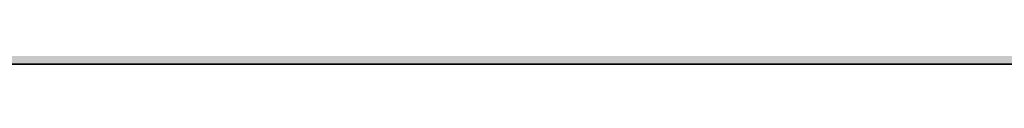
# Model space of a CAD drawing. Units: inches. Extents: x 2091 to 2899, y 967 to 2217.
# Tile 18 of 256: x 2312 to 2351, y 1091 to 1091. Entities that reach past the tile are written whole.
import ezdxf

# ---------------------------------------------------------------- set-up
doc = ezdxf.new("R2010")
doc.units = ezdxf.units.IN
doc.layers.add('A-WALL-PATT', color=141, linetype='Continuous', lineweight=13, true_color=0xadddf7)
doc.layers.add('C-PROP', color=7, linetype='Continuous', lineweight=35)

msp = doc.modelspace()

# ---------------------------------------------------------------- hatches: boundary and pattern name
at = {"layer": 'A-WALL-PATT'}
h = msp.add_hatch(color=256, dxfattribs=at)
h.dxf.hatch_style = 1
h.paths.add_polyline_path([(2212.144, 1941.419), (2387.644, 1941.419), (2387.644, 1824.419), (2392.144, 1824.419), (2392.144, 1941.419), (2609.644, 1941.419), (2609.644, 1825.919), (2614.144, 1825.919), (2614.144, 1941.419), (2794.144, 1941.419), (2794.144, 1928.762), (2803.144, 1928.762), (2803.144, 2050.919), (2203.144, 2050.919), (2203.144, 1900.758), (2212.144, 1900.758)])
h.paths.add_polyline_path([(2212.144, 1945.919), (2212.144, 2041.919), (2794.144, 2041.919), (2794.144, 1945.919), (2402.248, 1945.919), (2401.102, 1945.776), (2398.702, 1945.776)], flags=16)
h.paths.add_polyline_path([(2230.23, 1948.063), (2227.35, 1949.503), (2225.91, 1951.903), (2223.99, 1952.863), (2223.03, 1955.263), (2222.07, 1959.583), (2222.07, 1963.423), (2223.03, 1965.663), (2223.99, 1965.343), (2225.586, 1963.861), (2226.912, 1964.957), (2226.949, 1965.939), (2227.778, 1966.952), (2228.2, 1968.879), (2230.71, 1964.863), (2233.59, 1966.303), (2233.607, 1966.332), (2233.773, 1964.938), (2234.634, 1963.676), (2235.03, 1963.903), (2236.282, 1965.572), (2235.99, 1962.943), (2237.955, 1957.54), (2238.39, 1957.903), (2239.216, 1960.306), (2238.655, 1966.385), (2238.693, 1966.438), (2238.841, 1967.5), (2238.78, 1967.687), (2238.881, 1967.787), (2238.667, 1966.252), (2239.216, 1960.306), (2238.39, 1957.903), (2236.95, 1956.703), (2234.55, 1949.983)], flags=0)
h.paths.add_polyline_path([(2278.012, 1948.063), (2276.496, 1947.873), (2275.85, 1947.689), (2274.652, 1947.103)], flags=0)
h.paths.add_polyline_path([(2269.852, 1955.743), (2268.276, 1956.629), (2270.867, 1956.348), (2269.372, 1958.143), (2268.715, 1959.192), (2270.57, 1958.729), (2268.581, 1961.906), (2270.812, 1960.892), (2270.812, 1963.423), (2271.393, 1964.779), (2270.292, 1966.156), (2271.772, 1965.663), (2272.141, 1966.525), (2273.93, 1965.929), (2275.63, 1968.054), (2276.332, 1966.722), (2276.52, 1966.952), (2276.942, 1968.879), (2277.734, 1967.611), (2278.14, 1969.465), (2279.659, 1967.034), (2280.412, 1966.783), (2280.949, 1967.589), (2281.61, 1967.369), (2282.133, 1968.154), (2282.349, 1966.333), (2282.35, 1966.333), (2283.408, 1968.095), (2283.713, 1965.524), (2284.32, 1964.634), (2284.512, 1964.889), (2284.235, 1965.705), (2284.5, 1967.319), (2284.908, 1965.417), (2285.396, 1966.069), (2285.433, 1966.291), (2285.473, 1966.171), (2286.354, 1967.345), (2286.222, 1966.158), (2287.663, 1968.08), (2287.714, 1968.443), (2288.482, 1969.017), (2288.574, 1968.729), (2288.917, 1969.069), (2288.607, 1966.838), (2288.929, 1963.351), (2288.935, 1963.357), (2288.93, 1963.34), (2289.015, 1962.414), (2290.111, 1963.875), (2290.133, 1963.943), (2290.218, 1964.017), (2290.111, 1963.875), (2289.156, 1960.892), (2288.594, 1959.257), (2288.572, 1959.103), (2289.532, 1960.543), (2290.012, 1962.463), (2290.192, 1962.643), (2289.77, 1959.689), (2286.89, 1957.289), (2284.49, 1950.569), (2283.315, 1950.046), (2283.292, 1949.983), (2280.29, 1948.649), (2281.13, 1948.649), (2282.57, 1948.169), (2283.205, 1948.063), (2278.972, 1948.063), (2276.092, 1949.503), (2274.652, 1951.903), (2272.732, 1952.863)], flags=0)
h.paths.add_polyline_path([(2271.159, 1958.022), (2272.97, 1955.849), (2272.01, 1960.169), (2272.01, 1964.009), (2272.624, 1965.443), (2274.328, 1963.861), (2275.654, 1964.957), (2275.638, 1964.539), (2277.412, 1966.007), (2277.033, 1965.157), (2276.83, 1964.976), (2276.766, 1963.295), (2277.45, 1962.66), (2279.452, 1964.863), (2282.332, 1966.303), (2283.53, 1966.889), (2283.295, 1966.771), (2283.913, 1963.885), (2284.899, 1964.448), (2284.732, 1962.943), (2286.697, 1957.54), (2287.132, 1957.903), (2287.542, 1959.095), (2287.779, 1958.442), (2285.683, 1956.695), (2285.877, 1959.795), (2284.732, 1962.943), (2284.899, 1964.448), (2283.913, 1963.885), (2284.224, 1962.434), (2283.424, 1963.605), (2281.61, 1962.569), (2281.13, 1960.169), (2282.09, 1956.329), (2283.05, 1952.969), (2282.57, 1950.569), (2280.17, 1948.649), (2279.883, 1948.792), (2278.972, 1948.063), (2278.972, 1949.023), (2278.672, 1949.397), (2277.29, 1950.089), (2275.85, 1952.489), (2273.93, 1953.449), (2272.49, 1954.889), (2271.922, 1954.889), (2271.772, 1955.263)], flags=0)
h.paths.add_polyline_path([(2311.994, 1955.743), (2312.063, 1955.674), (2312.055, 1955.709)], flags=0)
h.paths.add_polyline_path([(2331.956, 1963.952), (2333.396, 1965.392), (2331.077, 1963.357), (2330.999, 1963.112)], flags=0)
h.paths.add_polyline_path([(2310.554, 1954.303), (2307.04, 1956.28), (2310.763, 1955.876), (2312.474, 1953.823), (2313.434, 1951.423), (2315.354, 1950.463), (2316.794, 1948.063), (2317.466, 1947.727), (2319.369, 1947.965), (2317.754, 1949.983), (2317.57, 1950.61), (2316.794, 1951.903), (2314.874, 1952.863), (2313.914, 1955.263), (2311.514, 1958.143), (2309.375, 1961.559), (2311.514, 1960.337), (2311.514, 1961.983), (2310.605, 1963.12), (2311.727, 1962.479), (2312.418, 1964.093), (2312.256, 1964.296), (2313.194, 1963.983), (2313.914, 1965.663), (2314.647, 1965.419), (2315.354, 1966.303), (2316.794, 1967.743), (2316.157, 1966.947), (2317.034, 1965.282), (2317.223, 1965.512), (2317.777, 1968.046), (2318.474, 1966.722), (2318.663, 1966.952), (2319.084, 1968.879), (2321.207, 1965.482), (2322.161, 1966.914), (2322.554, 1966.783), (2322.786, 1967.131), (2322.882, 1966.324), (2323.312, 1965.722), (2323.651, 1965.891), (2324.396, 1967.133), (2324.657, 1964.938), (2324.972, 1964.477), (2325.387, 1967.001), (2325.941, 1964.418), (2327.229, 1966.136), (2327.166, 1965.572), (2328.059, 1966.763), (2328.225, 1966.247), (2329.668, 1967.677), (2329.665, 1967.687), (2329.765, 1967.787), (2329.551, 1966.252), (2330.1, 1960.306), (2329.333, 1958.073), (2329.313, 1957.935), (2329.634, 1958.203), (2330.234, 1959.103), (2330.714, 1961.023), (2331.034, 1961.343), (2330.714, 1959.103), (2329.634, 1958.203), (2329.274, 1957.663), (2327.712, 1956.361), (2325.434, 1949.983), (2324.334, 1949.494), (2323.994, 1948.543), (2319.674, 1946.623), (2316.794, 1948.063), (2315.354, 1950.463), (2313.434, 1951.423)], flags=0)
h.paths.add_polyline_path([(2321.336, 1947.952), (2321.114, 1948.063), (2321.114, 1949.023), (2319.194, 1951.423), (2316.794, 1959.583), (2316.663, 1959.583), (2315.354, 1958.143), (2314.394, 1958.143), (2313.148, 1958.709), (2312.954, 1959.583), (2312.954, 1960.892), (2315.834, 1959.583), (2316.663, 1959.583), (2317.315, 1960.299), (2315.03, 1962.421), (2316.356, 1963.517), (2316.372, 1963.952), (2316.47, 1963.861), (2317.796, 1964.957), (2317.755, 1963.89), (2319.175, 1965.157), (2319.498, 1965.881), (2321.114, 1965.343), (2323.236, 1962.372), (2325.686, 1963.773), (2325.543, 1962.481), (2325.199, 1963.494), (2324.479, 1963.082), (2324.926, 1960.994), (2324.078, 1962.236), (2322.415, 1961.286), (2322.074, 1959.583), (2323.034, 1955.743), (2323.994, 1952.383), (2323.514, 1949.983), (2322.143, 1948.886), (2322.074, 1948.543)], flags=0)
h.paths.add_polyline_path([(2320.207, 1963.337), (2320.154, 1963.423), (2320.394, 1963.543)], flags=0)
h.paths.add_polyline_path([(2353.851, 1965.811), (2354.031, 1965.751), (2354.331, 1966.451), (2354.331, 1966.931)], flags=0)
h.paths.add_polyline_path([(2359.021, 1969.026), (2359.098, 1968.902), (2359.234, 1969.52), (2359.234, 1970)], flags=0)
h.paths.add_polyline_path([(2358.257, 1966.682), (2357.984, 1966.348), (2358.211, 1966.146), (2358.41, 1966.39)], flags=0)
h.paths.add_polyline_path([(2357.768, 1966.059), (2357.732, 1965.105), (2357.751, 1965.121), (2357.77, 1965.607), (2357.77, 1966.058)], flags=0)
h.paths.add_polyline_path([(2359.112, 1965.305), (2359.112, 1964.825), (2359.845, 1966.468), (2359.845, 1966.948)], flags=0)
h.paths.add_polyline_path([(2360.224, 1966.621), (2360.699, 1969.363), (2360.699, 1969.843), (2360.211, 1967.026), (2360.211, 1966.643)], flags=0)
h.paths.add_polyline_path([(2363.451, 1967.891), (2363.451, 1968.371), (2362.491, 1966.931), (2362.656, 1966.699)], flags=0)
h.paths.add_polyline_path([(2364.476, 1966.079), (2365.851, 1968.371), (2365.851, 1968.851), (2364.428, 1966.48)], flags=0)
h.paths.add_polyline_path([(2366.314, 1965.853), (2366.367, 1965.696), (2366.803, 1968.346), (2366.803, 1968.826)], flags=0)
h.paths.add_polyline_path([(2367.165, 1965.804), (2367.291, 1966.931), (2367.291, 1967.411), (2367.103, 1965.72)], flags=0)
h.paths.add_polyline_path([(2370.037, 1959.974), (2371.014, 1963.025), (2371.014, 1963.505), (2370.037, 1960.454)], flags=0)
h.paths.add_polyline_path([(2371.611, 1960.211), (2372.571, 1961.651), (2372.571, 1962.131), (2371.803, 1960.979)], flags=0)
h.paths.add_polyline_path([(2350.874, 1956.005), (2351.931, 1955.891), (2354.491, 1953.331), (2353.851, 1954.931), (2351.451, 1957.811), (2347.936, 1963.426), (2347.936, 1963.906), (2351.451, 1958.291), (2353.705, 1955.585), (2352.891, 1959.251), (2352.891, 1959.731), (2352.891, 1961.925), (2356.731, 1959.731), (2358.454, 1961.627), (2354.811, 1965.011), (2355.031, 1965.286), (2358.691, 1961.887), (2361.531, 1965.011), (2364.376, 1966.433), (2364.524, 1965.187), (2365.454, 1963.824), (2365.881, 1964.068), (2365.371, 1966.451), (2365.371, 1966.931), (2366.811, 1960.211), (2366.811, 1959.731), (2366.389, 1952.981), (2367.771, 1956.851), (2368.641, 1957.576), (2366.811, 1962.611), (2366.811, 1963.091), (2368.775, 1957.688), (2369.211, 1958.051), (2370.002, 1960.352), (2369.475, 1966.053), (2369.513, 1966.106), (2369.514, 1966.111), (2369.475, 1966.533), (2369.513, 1966.586), (2369.615, 1967.313), (2369.183, 1968.659), (2369.183, 1969.139), (2369.601, 1967.835), (2369.701, 1967.934), (2369.718, 1968.055), (2370.145, 1968.374), (2369.779, 1968.011), (2369.701, 1967.454), (2370.468, 1968.214), (2369.675, 1967.266), (2369.514, 1966.111), (2370.037, 1960.454), (2370.037, 1959.974), (2369.442, 1958.243), (2370.651, 1959.251), (2371.046, 1962.018), (2371.131, 1962.131), (2370.651, 1958.771), (2367.771, 1956.371), (2365.371, 1949.651), (2362.079, 1948.188), (2363.451, 1947.731), (2361.051, 1947.731), (2360.091, 1947.731), (2357.104, 1947.357), (2360.091, 1948.211), (2358.171, 1949.171), (2356.731, 1951.571), (2354.811, 1952.531), (2351.931, 1955.411)], flags=0)
h.paths.add_polyline_path([(2361.051, 1948.691), (2359.131, 1951.091), (2356.731, 1959.251), (2355.771, 1959.251), (2352.891, 1960.56), (2352.891, 1961.445), (2355.891, 1959.731), (2356.731, 1959.731), (2356.837, 1959.368), (2361.531, 1964.531), (2363.248, 1965.389), (2364.925, 1963.042), (2362.491, 1961.651), (2362.064, 1959.517), (2362.971, 1955.891), (2363.931, 1952.531), (2363.931, 1952.051), (2363.451, 1949.651), (2361.051, 1947.731)], flags=0)
h.paths.add_polyline_path([(2359.131, 1951.571), (2359.291, 1951.371), (2361.051, 1954.451), (2361.051, 1954.931)], flags=0)
h.paths.add_polyline_path([(2357.22, 1966.546), (2356.793, 1968.815), (2356.793, 1969.295), (2357.22, 1967.026)], flags=0)
h.paths.add_polyline_path([(2361.051, 1954.451), (2361.531, 1958.771), (2361.531, 1959.251), (2361.051, 1954.931)], flags=0)
h.paths.add_polyline_path([(2402.548, 1948.486), (2402.302, 1948.416), (2402.59, 1948.416)], flags=0)
h.paths.add_polyline_path([(2394.142, 1956.096), (2395.685, 1954.553), (2396.72, 1953.971), (2396.062, 1955.616), (2395.241, 1956.601), (2395.879, 1956.442), (2395.102, 1959.936), (2395.102, 1963.776), (2396.062, 1966.016), (2397.022, 1965.696), (2398.618, 1964.214), (2399.944, 1965.31), (2399.981, 1966.292), (2400.811, 1967.305), (2401.232, 1969.232), (2403.538, 1965.543), (2403.942, 1967.389), (2404.702, 1967.136), (2405.46, 1966.075), (2406.622, 1966.656), (2406.64, 1966.685), (2406.805, 1965.291), (2406.926, 1965.115), (2407.342, 1964.976), (2407.874, 1965.774), (2408.169, 1964.398), (2409.315, 1965.925), (2409.217, 1965.051), (2409.445, 1963.131), (2410.306, 1961.87), (2410.702, 1962.096), (2411.442, 1963.082), (2411.165, 1963.898), (2411.616, 1966.64), (2411.725, 1966.791), (2411.873, 1967.853), (2411.813, 1968.041), (2411.913, 1968.14), (2411.699, 1966.605), (2412.248, 1960.659), (2413.225, 1963.71), (2414.378, 1964.721), (2414.513, 1965.693), (2414.453, 1965.881), (2414.553, 1965.98), (2414.378, 1964.721), (2414.52, 1964.846), (2414.365, 1964.631), (2414.339, 1964.445), (2414.888, 1958.499), (2414.062, 1956.096), (2412.622, 1954.896), (2410.171, 1948.033), (2410.017, 1948.084), (2405.902, 1946.256), (2405.902, 1947.216), (2405.204, 1948.089), (2404.222, 1948.416), (2403.262, 1948.416), (2400.382, 1949.856), (2399.662, 1951.056), (2397.982, 1952.736), (2397.022, 1953.216), (2395.685, 1954.553), (2392.657, 1956.257)], flags=0)
h.paths.add_polyline_path([(2409.086, 1964.407), (2409.13, 1964.276), (2409.262, 1964.496)], flags=0)
h.paths.add_polyline_path([(2397.742, 1961.616), (2398.702, 1963.856), (2399.662, 1963.536), (2401.427, 1965.741), (2401.791, 1966.559), (2402.071, 1965.071), (2402.836, 1964.393), (2403.262, 1964.915), (2403.338, 1964.771), (2402.616, 1963.976), (2402.499, 1960.902), (2403.543, 1959.932), (2404.413, 1960.89), (2404.702, 1962.336), (2407.916, 1964.172), (2409.52, 1961.927), (2410.987, 1957.893), (2411.422, 1958.256), (2412.048, 1960.076), (2412.41, 1959.079), (2411.676, 1958.467), (2411.662, 1958.256), (2411.626, 1958.426), (2409.982, 1957.056), (2407.582, 1950.336), (2403.262, 1948.416), (2403.262, 1949.376), (2401.342, 1951.776), (2399.417, 1958.324), (2397.742, 1959.085), (2397.742, 1959.97), (2397.102, 1960.336), (2397.742, 1960.045)], flags=0)
h.paths.add_polyline_path([(2405.902, 1952.976), (2405.95, 1953.408), (2406.017, 1953.176)], flags=0)
h.paths.add_polyline_path([(2449.818, 1967.114), (2449.752, 1967.136), (2449.794, 1967.078)], flags=0)
h.paths.add_polyline_path([(2451.698, 1966.618), (2451.741, 1966.69), (2451.692, 1966.666)], flags=0)
h.paths.add_polyline_path([(2454.344, 1965.738), (2455.752, 1967.616), (2455.992, 1968.096), (2454.364, 1965.925)], flags=0)
h.paths.add_polyline_path([(2457.547, 1968.864), (2457.787, 1969.344), (2457.054, 1968.796), (2457.008, 1968.46)], flags=0)
h.paths.add_polyline_path([(2456.922, 1967.857), (2456.802, 1968.229), (2456.723, 1967.66)], flags=0)
h.paths.add_polyline_path([(2457.302, 1967.377), (2457.542, 1967.857), (2456.81, 1966.84), (2456.741, 1966.7), (2456.749, 1966.608)], flags=0)
h.paths.add_polyline_path([(2458.275, 1963.71), (2458.155, 1963.335), (2460.354, 1965.265), (2460.594, 1965.745)], flags=0)
h.paths.add_polyline_path([(2458.392, 1962.816), (2458.364, 1962.618), (2459.592, 1964.256), (2459.832, 1964.736)], flags=0)
h.paths.add_polyline_path([(2459.352, 1962.816), (2459.272, 1962.496), (2460.072, 1963.296), (2460.312, 1963.776)], flags=0)
h.paths.add_polyline_path([(2458.68, 1960.608), (2458.632, 1960.416), (2459.592, 1961.856), (2459.832, 1962.336)], flags=0)
h.paths.add_polyline_path([(2437.838, 1956.243), (2439.192, 1956.096), (2441.352, 1953.936), (2440.872, 1955.136), (2438.472, 1958.016), (2438.072, 1958.656), (2438.712, 1958.496), (2440.64, 1956.183), (2439.912, 1959.456), (2439.912, 1963.296), (2441.352, 1966.656), (2441.592, 1967.136), (2441.112, 1966.016), (2442.072, 1965.696), (2443.989, 1968.092), (2444.241, 1966.751), (2444.917, 1966.152), (2445.677, 1967.08), (2446.255, 1969.725), (2446.495, 1970.205), (2446.282, 1969.232), (2447.363, 1967.503), (2447.72, 1969.568), (2447.96, 1970.048), (2447.485, 1967.307), (2448.792, 1965.216), (2448.472, 1964.864), (2448.552, 1964.736), (2451.452, 1966.186), (2451.615, 1964.811), (2452.308, 1963.796), (2453.235, 1964.326), (2454.072, 1960.416), (2453.629, 1953.318), (2454.792, 1956.576), (2455.032, 1957.056), (2455.719, 1957.628), (2453.832, 1962.816), (2453.941, 1963.794), (2453.335, 1965.578), (2453.824, 1968.551), (2454.064, 1969.031), (2453.575, 1966.058), (2454.04, 1964.688), (2453.832, 1962.816), (2455.719, 1957.628), (2456.367, 1958.168), (2457.058, 1960.179), (2457.298, 1960.659), (2456.472, 1958.256), (2457.718, 1959.294), (2457.672, 1958.976), (2454.89, 1956.657), (2453.614, 1953.085), (2453.592, 1952.736), (2453.352, 1952.256), (2453.36, 1952.372), (2452.632, 1950.336), (2452.392, 1949.856), (2449.204, 1948.439), (2450.712, 1947.936), (2448.072, 1947.936), (2447.112, 1947.936), (2444.552, 1947.616), (2447.2, 1948.372), (2445.192, 1949.376), (2443.752, 1951.776), (2441.832, 1952.736), (2438.952, 1955.616)], flags=0)
h.paths.add_polyline_path([(2443.992, 1959.936), (2444.04, 1959.773), (2444.122, 1959.862)], flags=0)
h.paths.add_polyline_path([(2442.912, 1959.936), (2443.032, 1959.936), (2442.446, 1960.202)], flags=0)
h.paths.add_polyline_path([(2444.983, 1965.02), (2445.279, 1965.265), (2445.519, 1965.745), (2444.994, 1965.31)], flags=0)
h.paths.add_polyline_path([(2446.133, 1965.03), (2446.33, 1965.471), (2444.97, 1964.258), (2444.73, 1963.778)], flags=0)
h.paths.add_polyline_path([(2442.792, 1959.456), (2443.752, 1959.456), (2446.152, 1951.296), (2446.412, 1951.751), (2446.392, 1951.776), (2448.081, 1954.73), (2448.552, 1958.976), (2441.832, 1965.216), (2442.155, 1965.619), (2448.792, 1959.456), (2448.312, 1955.136), (2448.072, 1954.656), (2446.412, 1951.751), (2448.312, 1949.376), (2448.312, 1948.416), (2450.541, 1950.199), (2450.952, 1952.256), (2449.992, 1955.616), (2449.032, 1959.456), (2449.512, 1961.856), (2449.752, 1962.336), (2449.675, 1961.949), (2452.995, 1963.846), (2453.064, 1963.519), (2452.885, 1963.783), (2449.675, 1961.949), (2449.272, 1959.936), (2450.232, 1956.096), (2451.192, 1952.736), (2450.712, 1950.336), (2450.472, 1949.856), (2448.072, 1947.936), (2448.072, 1948.536), (2445.432, 1949.856), (2443.992, 1952.256), (2442.072, 1953.216), (2441.112, 1955.616), (2440.152, 1959.936), (2440.152, 1960.656)], flags=0)
h.paths.add_polyline_path([(2456.692, 1966.986), (2457.608, 1968.081), (2457.848, 1968.561), (2456.932, 1967.466)], flags=0)
h.paths.add_polyline_path([(2489.897, 1966.58), (2489.943, 1966.189), (2490.747, 1967.53), (2491.319, 1968.951)], flags=0)
h.paths.add_polyline_path([(2473.562, 1956.407), (2477.14, 1956.019), (2476.955, 1956.241), (2475.108, 1957.28), (2476.347, 1956.97), (2475.187, 1958.824), (2476.919, 1958.391), (2475.412, 1960.799), (2477.787, 1959.719), (2477.787, 1962.25), (2477.637, 1962.438), (2477.823, 1962.332), (2478.359, 1963.584), (2478.359, 1963.671), (2477.324, 1964.965), (2478.715, 1964.501), (2479.319, 1965.911), (2480.279, 1965.591), (2481.784, 1967.472), (2482.116, 1965.705), (2482.881, 1965.028), (2483.209, 1965.429), (2483.22, 1965.715), (2483.076, 1965.989), (2483.712, 1966.766), (2484.13, 1968.679), (2484.702, 1970.1), (2484.489, 1969.127), (2486.503, 1965.905), (2487.387, 1965.61), (2488.153, 1966.759), (2488.717, 1965.97), (2489.2, 1966.212), (2489.331, 1965.111), (2490.394, 1963.622), (2490.661, 1963.775), (2490.494, 1964.554), (2490.923, 1963.925), (2491.319, 1964.151), (2491.333, 1964.17), (2491.21, 1964.532), (2491.282, 1964.966), (2491.426, 1964.293), (2494.076, 1967.828), (2494.498, 1966.515), (2494.598, 1966.614), (2494.689, 1967.27), (2495.107, 1967.582), (2495.13, 1967.748), (2495.07, 1967.936), (2495.17, 1968.035), (2495.032, 1967.044), (2495.754, 1967.759), (2494.982, 1966.686), (2494.956, 1966.5), (2495.479, 1960.837), (2495.91, 1962.184), (2496.482, 1963.605), (2496.073, 1962.327), (2496.769, 1962.938), (2496.599, 1962.711), (2496.119, 1959.351), (2496.733, 1960.272), (2496.987, 1961.29), (2497.559, 1962.711), (2497.079, 1960.791), (2496.507, 1959.37), (2495.547, 1957.93), (2492.759, 1955.606), (2490.839, 1950.231), (2490.267, 1948.81), (2485.947, 1946.89), (2483.067, 1948.33), (2481.627, 1950.73), (2479.707, 1951.69), (2476.827, 1954.57)], flags=0)
h.paths.add_polyline_path([(2485.577, 1948.313), (2485.559, 1948.311), (2485.579, 1948.311)], flags=0)
h.paths.add_polyline_path([(2478.645, 1954.551), (2478.109, 1956.963), (2479.319, 1955.511), (2480.279, 1953.111), (2482.199, 1952.151), (2483.639, 1949.751), (2486.519, 1948.311), (2486.519, 1949.271), (2484.739, 1951.496), (2484.027, 1950.25), (2481.627, 1958.41), (2482.375, 1959.233), (2482.199, 1959.831), (2483.198, 1960.929), (2479.707, 1964.17), (2480.603, 1965.29), (2481.875, 1964.109), (2482.666, 1964.764), (2482.615, 1963.422), (2482.989, 1963.075), (2484.008, 1963.984), (2484.684, 1965.498), (2484.58, 1965.405), (2485.357, 1967.147), (2485.121, 1965.781), (2486.427, 1963.69), (2488.145, 1964.549), (2489.822, 1962.202), (2490.747, 1962.73), (2492, 1964.4), (2492.076, 1965.087), (2492.213, 1964.684), (2492.485, 1965.047), (2492.279, 1963.191), (2494.244, 1957.788), (2494.563, 1958.054), (2494.933, 1959.133), (2495.505, 1960.554), (2494.679, 1958.151), (2494.107, 1956.73), (2494.563, 1958.054), (2493.409, 1957.092), (2491.707, 1961.77), (2492, 1964.4), (2490.747, 1962.73), (2487.712, 1960.996), (2487.479, 1959.831), (2488.439, 1955.991), (2489.399, 1952.631), (2488.919, 1950.231), (2488.577, 1949.957), (2488.347, 1948.81), (2487.652, 1948.254), (2487.479, 1948.311), (2486.519, 1948.311), (2483.639, 1949.751), (2482.199, 1952.151), (2480.279, 1953.111), (2478.839, 1954.551)], flags=0)
h.paths.add_polyline_path([(2526.648, 1966.988), (2526.517, 1967.031), (2526.6, 1966.915)], flags=0)
h.paths.add_polyline_path([(2528.471, 1966.447), (2528.574, 1966.62), (2528.457, 1966.561)], flags=0)
h.paths.add_polyline_path([(2534.133, 1967.496), (2534.157, 1967.543), (2534.06, 1967.408)], flags=0)
h.paths.add_polyline_path([(2536.162, 1964.051), (2535.157, 1962.711), (2535.101, 1962.316), (2536.117, 1963.671), (2536.421, 1964.278)], flags=0)
h.paths.add_polyline_path([(2535.157, 1959.831), (2536.117, 1961.271), (2536.597, 1962.231), (2535.253, 1960.215)], flags=0)
h.paths.add_polyline_path([(2513.249, 1956.285), (2516.221, 1955.963), (2514.997, 1957.431), (2514.196, 1958.712), (2515.477, 1958.391), (2516.932, 1956.646), (2516.437, 1958.871), (2516.437, 1962.711), (2516.873, 1963.727), (2515.346, 1965.635), (2517.397, 1964.951), (2517.877, 1966.071), (2518.357, 1967.031), (2517.877, 1965.911), (2518.837, 1965.591), (2520.487, 1967.653), (2520.766, 1966.166), (2521.53, 1965.489), (2521.781, 1965.795), (2521.801, 1966.307), (2521.478, 1966.921), (2521.246, 1967.126), (2521.178, 1967.491), (2521.478, 1966.921), (2522.01, 1966.449), (2522.257, 1966.75), (2522.78, 1969.14), (2523.26, 1970.1), (2523.047, 1969.127), (2524.673, 1966.526), (2526.037, 1966.071), (2526.795, 1965.01), (2527.977, 1965.601), (2528.14, 1964.227), (2528.665, 1963.458), (2529.389, 1963.872), (2529.33, 1964.147), (2529.481, 1963.925), (2529.877, 1964.151), (2529.984, 1964.293), (2529.789, 1965.203), (2530.062, 1964.398), (2532.802, 1968.051), (2533.148, 1966.976), (2533.248, 1967.075), (2533.339, 1967.731), (2533.673, 1967.98), (2533.728, 1968.035), (2533.514, 1966.5), (2534.025, 1960.972), (2534.56, 1962.645), (2535.04, 1963.605), (2534.063, 1960.554), (2533.237, 1958.151), (2534.288, 1959.027), (2534.197, 1958.391), (2531.513, 1956.154), (2529.397, 1950.231), (2528.917, 1949.271), (2526.449, 1948.174), (2527.477, 1947.831), (2530.357, 1947.351), (2524.597, 1947.351), (2521.717, 1948.791), (2520.277, 1951.191), (2518.357, 1952.151), (2515.477, 1955.031)], flags=0)
h.paths.add_polyline_path([(2523.935, 1967.19), (2523.62, 1966.484), (2523.77, 1966.242)], flags=0)
h.paths.add_polyline_path([(2518.837, 1953.111), (2517.877, 1955.511), (2516.885, 1959.977), (2516.917, 1959.962), (2516.917, 1962.025), (2520.757, 1959.831), (2522.025, 1961.226), (2518.357, 1964.631), (2519.003, 1965.438), (2520.433, 1964.109), (2521.301, 1964.827), (2521.245, 1963.355), (2525.638, 1959.276), (2526.037, 1961.271), (2529.397, 1963.191), (2530.65, 1964.861), (2530.665, 1964.998), (2530.692, 1964.917), (2531.088, 1965.445), (2530.946, 1964.169), (2530.692, 1964.917), (2529.397, 1963.191), (2526.363, 1961.457), (2526.037, 1959.831), (2526.997, 1955.991), (2527.957, 1952.631), (2527.477, 1950.231), (2527.134, 1949.957), (2526.974, 1949.154), (2526.697, 1949.031), (2524.597, 1947.351), (2524.597, 1948.311), (2524.277, 1948.711), (2522.197, 1949.751), (2520.757, 1952.151)], flags=0)
h.paths.add_polyline_path([(2520.277, 1958.871), (2520.853, 1959.505), (2523.157, 1951.671), (2524.614, 1954.22), (2524.597, 1954.071), (2522.677, 1950.711)], flags=0)
h.paths.add_polyline_path([(2559.371, 1966.311), (2559.398, 1966.325), (2559.402, 1966.345)], flags=0)
h.paths.add_polyline_path([(2549.771, 1957.191), (2552.651, 1954.311), (2552.134, 1955.603), (2550.611, 1957.431), (2547.096, 1963.046), (2545.776, 1965.206), (2549.291, 1959.591), (2551.691, 1956.711), (2550.793, 1960.752), (2550.731, 1960.78), (2550.731, 1964.871), (2551.691, 1967.111), (2552.651, 1966.791), (2554.247, 1965.309), (2555.034, 1965.96), (2555.582, 1966.645), (2555.61, 1967.387), (2556.439, 1968.401), (2556.861, 1970.327), (2559.371, 1966.311), (2560.691, 1964.151), (2562.409, 1965.01), (2561.651, 1966.071), (2560.331, 1968.231), (2561.758, 1966.233), (2562.347, 1967.116), (2562.434, 1966.387), (2563.128, 1965.37), (2563.571, 1965.591), (2563.588, 1965.62), (2563.363, 1967.524), (2563.722, 1965.844), (2565.06, 1968.073), (2564.733, 1965.129), (2565.118, 1963.333), (2567.445, 1966.436), (2567.316, 1967.833), (2567.354, 1967.886), (2567.502, 1968.948), (2567.441, 1969.136), (2567.542, 1969.235), (2567.328, 1967.7), (2567.877, 1961.754), (2568.747, 1964.47), (2568.636, 1965.673), (2568.674, 1965.726), (2568.822, 1966.788), (2568.761, 1966.976), (2568.862, 1967.075), (2568.648, 1965.54), (2568.726, 1964.693), (2568.854, 1964.805), (2568.747, 1964.47), (2568.817, 1963.706), (2568.971, 1963.911), (2568.866, 1963.177), (2569.197, 1959.594), (2568.371, 1957.191), (2566.931, 1955.991), (2564.62, 1949.521), (2564.651, 1949.511), (2564.617, 1949.511), (2564.531, 1949.271), (2560.211, 1947.351), (2557.331, 1948.791), (2556.045, 1950.934), (2556.011, 1950.951), (2555.857, 1951.208), (2553.971, 1952.151), (2551.091, 1955.031), (2546.65, 1957.53)], flags=0)
h.paths.add_polyline_path([(2567.026, 1959.33), (2567.035, 1959.305), (2567.051, 1959.351)], flags=0)
h.paths.add_polyline_path([(2551.968, 1962.518), (2553.011, 1964.951), (2553.971, 1964.631), (2555.567, 1963.149), (2556.893, 1964.246), (2556.93, 1965.227), (2557.144, 1965.489), (2556.42, 1966.131), (2556.391, 1966.105), (2556.38, 1966.166), (2556.42, 1966.131), (2556.952, 1966.605), (2557.092, 1966.919), (2557.571, 1966.01), (2557.759, 1966.241), (2557.418, 1964.68), (2556.893, 1964.246), (2556.807, 1961.998), (2560.691, 1958.391), (2560.636, 1957.893), (2560.811, 1957.191), (2561.771, 1953.831), (2561.291, 1951.431), (2559.11, 1949.687), (2559.156, 1949.629), (2563.027, 1951.349), (2562.611, 1949.271), (2560.211, 1947.351), (2560.211, 1948.311), (2559.251, 1949.511), (2558.891, 1949.511), (2558.891, 1949.961), (2558.291, 1950.711), (2558.054, 1951.518), (2556.971, 1952.871), (2555.068, 1959.341), (2552.051, 1961.065), (2552.051, 1962.471)], flags=0)
h.paths.add_polyline_path([(2588.33, 1958.391), (2588.61, 1958.111), (2588.553, 1958.367)], flags=0)
h.paths.add_polyline_path([(2594.745, 1950.493), (2593.958, 1953.172), (2593.13, 1954.551), (2591.21, 1955.511), (2590.25, 1957.911), (2588.309, 1960.24), (2586.177, 1961.209), (2587.85, 1960.791), (2587.253, 1961.744), (2588.441, 1961.065), (2588.441, 1962.656), (2588.422, 1962.665), (2588.441, 1962.711), (2586.914, 1964.62), (2588.877, 1963.728), (2589.29, 1964.692), (2589.29, 1966.071), (2590.25, 1968.311), (2591.21, 1967.991), (2592.806, 1966.509), (2594.132, 1967.606), (2594.169, 1968.587), (2594.999, 1969.601), (2595.42, 1971.527), (2597.93, 1967.511), (2600.81, 1968.951), (2600.827, 1968.98), (2600.993, 1967.587), (2601.854, 1966.325), (2602.107, 1966.47), (2602.236, 1967.255), (2602.357, 1966.693), (2603.502, 1968.221), (2603.21, 1965.591), (2605.175, 1960.188), (2605.507, 1960.465), (2605.026, 1965.673), (2605.064, 1965.726), (2605.212, 1966.788), (2605.152, 1966.976), (2605.252, 1967.075), (2605.343, 1967.731), (2605.953, 1968.187), (2605.875, 1969.033), (2605.913, 1969.086), (2606.061, 1970.148), (2606, 1970.336), (2606.101, 1970.435), (2605.887, 1968.9), (2606.436, 1962.954), (2605.61, 1960.551), (2605.997, 1960.874), (2606.564, 1962.645), (2608.241, 1964.117), (2608.01, 1963.191), (2607.05, 1961.751), (2606.631, 1961.402), (2606.201, 1958.391), (2603.321, 1955.991), (2600.921, 1949.271), (2596.601, 1947.351), (2593.721, 1948.791), (2592.857, 1950.231), (2592.65, 1950.231)], flags=0)
h.paths.add_polyline_path([(2596.601, 1947.351), (2596.601, 1948.311), (2594.681, 1950.711), (2596.155, 1953.29), (2595.53, 1954.071), (2593.199, 1961.996), (2592.651, 1962.505), (2591.78, 1963.003), (2593.283, 1964.246), (2593.32, 1965.227), (2594.15, 1966.241), (2594.571, 1968.167), (2596.183, 1965.589), (2596.951, 1966.435), (2598.041, 1966.071), (2598.799, 1965.01), (2599.961, 1965.591), (2599.979, 1965.62), (2600.144, 1964.227), (2601.005, 1962.965), (2601.401, 1963.191), (2602.653, 1964.861), (2602.361, 1962.231), (2603.793, 1958.295), (2601.978, 1953.212), (2601.946, 1952.709), (2599.469, 1951.608), (2599.001, 1949.271)], flags=0)
h.paths.add_polyline_path([(2597.561, 1958.871), (2597.671, 1959.419), (2597.595, 1958.736)], flags=0)
h.paths.add_polyline_path([(2623.666, 1961.254), (2625.519, 1960.791), (2624.966, 1961.676), (2627.199, 1960.66), (2627.199, 1961.151), (2626.959, 1962.231), (2626.959, 1963.491), (2625.582, 1965.212), (2626.959, 1964.425), (2626.959, 1965.831), (2626.869, 1965.861), (2627.919, 1968.311), (2628.879, 1967.991), (2630.475, 1966.509), (2631.801, 1967.606), (2631.838, 1968.587), (2632.668, 1969.601), (2633.089, 1971.527), (2635.599, 1967.511), (2638.479, 1968.951), (2638.497, 1968.98), (2638.662, 1967.587), (2639.176, 1966.833), (2639.78, 1967.84), (2640.026, 1966.693), (2641.171, 1968.221), (2640.879, 1965.591), (2641.114, 1964.945), (2641.411, 1965.341), (2641.308, 1964.412), (2642.844, 1960.188), (2643.279, 1960.551), (2644.085, 1962.895), (2643.784, 1966.153), (2643.807, 1966.185), (2643.601, 1968.418), (2643.523, 1968.661), (2643.73, 1970.148), (2643.67, 1970.336), (2643.77, 1970.435), (2643.556, 1968.9), (2643.601, 1968.418), (2643.91, 1967.456), (2644.01, 1967.555), (2643.812, 1966.132), (2644.105, 1962.954), (2644.239, 1961.351), (2644.719, 1961.751), (2645.033, 1962.222), (2645.322, 1963.125), (2646.076, 1963.787), (2645.033, 1962.222), (2644.345, 1960.074), (2643.519, 1957.671), (2642.079, 1956.471), (2639.72, 1949.864), (2639.876, 1949.838), (2635.359, 1947.831), (2632.479, 1949.271), (2631.039, 1951.671), (2629.119, 1952.631), (2628.159, 1955.031), (2625.759, 1957.911)], flags=0)
h.paths.add_polyline_path([(2627.816, 1956.574), (2627.374, 1958.566), (2626.376, 1959.763), (2627.199, 1959.351), (2627.374, 1958.566), (2627.919, 1957.911), (2628.879, 1955.511), (2630.799, 1954.551), (2632.239, 1952.151), (2633.315, 1951.613), (2631.039, 1959.351), (2631.498, 1959.856), (2630.799, 1962.231), (2631.45, 1962.947), (2630.715, 1963.629), (2632.041, 1964.726), (2632.078, 1965.707), (2632.292, 1965.969), (2631.705, 1966.489), (2633.136, 1967.766), (2633.329, 1968.647), (2634.675, 1966.494), (2635.208, 1967.081), (2636.799, 1966.551), (2637.676, 1967.867), (2638.994, 1966.022), (2639.705, 1966.429), (2641.119, 1959.831), (2640.93, 1956.806), (2639.439, 1952.631), (2638.227, 1952.093), (2637.759, 1949.751), (2635.359, 1947.831), (2635.359, 1948.791), (2633.439, 1951.191), (2633.315, 1951.613), (2632.239, 1952.151), (2630.799, 1954.551), (2628.879, 1955.511)], flags=0)
h.paths.add_polyline_path([(2637.759, 1953.831), (2637.279, 1955.511), (2636.319, 1959.351), (2636.799, 1961.751), (2639.234, 1963.142), (2637.557, 1965.49), (2638.739, 1966.081), (2638.902, 1964.707), (2639.763, 1963.445), (2636.799, 1961.751), (2636.532, 1960.418), (2637.039, 1958.391), (2637.999, 1955.031)], flags=0)
h.paths.add_polyline_path([(2668.567, 1951.431), (2667.607, 1953.831), (2665.207, 1956.711), (2662.294, 1961.365), (2665.447, 1959.591), (2666.647, 1958.391), (2666.647, 1959.975), (2666.058, 1960.682), (2666.647, 1960.345), (2666.647, 1961.991), (2666.7, 1962.114), (2666.407, 1963.431), (2666.407, 1967.271), (2667.367, 1969.511), (2668.327, 1969.191), (2669.923, 1967.709), (2671.249, 1968.806), (2671.286, 1969.787), (2672.116, 1970.801), (2672.537, 1972.727), (2675.047, 1968.711), (2677.927, 1970.151), (2677.945, 1970.18), (2678.11, 1968.787), (2678.971, 1967.525), (2679.367, 1967.751), (2680.62, 1969.421), (2680.327, 1966.791), (2682.292, 1961.388), (2682.727, 1961.751), (2683.358, 1963.587), (2683.232, 1964.953), (2683.27, 1965.006), (2683.393, 1965.889), (2683.36, 1966.249), (2683.358, 1966.256), (2683.359, 1966.257), (2682.992, 1970.233), (2683.03, 1970.286), (2683.178, 1971.348), (2683.118, 1971.536), (2683.218, 1971.635), (2683.004, 1970.1), (2683.359, 1966.257), (2683.458, 1966.355), (2683.393, 1965.889), (2683.414, 1965.665), (2684.424, 1966.872), (2683.553, 1964.154), (2683.358, 1963.587), (2683.793, 1958.874), (2682.967, 1956.471), (2681.527, 1955.271), (2680.109, 1951.3), (2680.085, 1950.912), (2679.977, 1950.93), (2679.127, 1948.551), (2674.807, 1946.631), (2671.927, 1948.071), (2670.487, 1950.471)], flags=0)
h.paths.add_polyline_path([(2671.936, 1953.227), (2671.687, 1953.351), (2670.247, 1955.751), (2668.327, 1956.711), (2667.357, 1959.138), (2669.527, 1958.151), (2670.487, 1958.151), (2671.479, 1959.242), (2670.684, 1961.945), (2668.89, 1963.612), (2667.307, 1964.331), (2668.567, 1963.911), (2668.831, 1964.241), (2670.247, 1963.431), (2672.422, 1965.823), (2672.777, 1967.447), (2673.234, 1966.716), (2674.412, 1968.012), (2673.981, 1965.522), (2675.287, 1963.431), (2675.554, 1963.564), (2675.932, 1965.456), (2676.247, 1965.351), (2677.005, 1964.29), (2678.167, 1964.871), (2679.607, 1967.271), (2680.327, 1963.911), (2680.307, 1963.577), (2680.347, 1963.458), (2680.86, 1964.141), (2680.567, 1961.511), (2681.104, 1960.037), (2678.887, 1953.831), (2677.092, 1953.033), (2677.687, 1950.951), (2677.207, 1948.551), (2674.807, 1946.631), (2674.807, 1947.591), (2672.887, 1949.991)], flags=0)
h.paths.add_polyline_path([(2673.985, 1951.911), (2674.567, 1952.931), (2674.567, 1951.911), (2676.967, 1953.831), (2677.447, 1956.231), (2676.487, 1959.591), (2676.247, 1960.551), (2679.73, 1962.541), (2680.059, 1961.002), (2679.211, 1962.245), (2676.247, 1960.551), (2676.487, 1959.591), (2677.447, 1956.231), (2676.967, 1953.831), (2674.567, 1951.911)], flags=0)
h.paths.add_polyline_path([(2707.479, 1952.815), (2706.519, 1955.215), (2705.559, 1959.535), (2705.559, 1963.375), (2706.519, 1965.615), (2707.479, 1965.295), (2709.075, 1963.813), (2710.401, 1964.909), (2710.438, 1965.891), (2711.268, 1966.904), (2711.689, 1968.831), (2714.199, 1964.815), (2717.079, 1966.255), (2717.097, 1966.284), (2717.262, 1964.89), (2718.123, 1963.628), (2718.519, 1963.855), (2719.771, 1965.524), (2719.479, 1962.895), (2721.444, 1957.492), (2721.879, 1957.855), (2722.705, 1960.258), (2722.144, 1966.337), (2722.182, 1966.39), (2722.33, 1967.452), (2722.27, 1967.639), (2722.37, 1967.739), (2722.156, 1966.204), (2722.705, 1960.258), (2721.879, 1957.855), (2720.439, 1956.655), (2718.039, 1949.935), (2713.719, 1948.015), (2710.839, 1949.455), (2709.399, 1951.855)], flags=0)
h.paths.add_polyline_path([(2749.301, 1952.815), (2748.341, 1955.215), (2747.381, 1959.535), (2747.381, 1963.375), (2748.341, 1965.615), (2749.301, 1965.295), (2750.897, 1963.813), (2752.223, 1964.909), (2752.26, 1965.891), (2753.09, 1966.904), (2753.511, 1968.831), (2756.021, 1964.815), (2758.901, 1966.255), (2758.919, 1966.284), (2759.084, 1964.89), (2759.945, 1963.628), (2760.341, 1963.855), (2761.593, 1965.524), (2761.301, 1962.895), (2763.266, 1957.492), (2763.701, 1957.855), (2764.527, 1960.258), (2763.966, 1966.337), (2764.004, 1966.39), (2764.152, 1967.452), (2764.092, 1967.639), (2764.192, 1967.739), (2763.978, 1966.204), (2764.527, 1960.258), (2763.701, 1957.855), (2762.261, 1956.655), (2759.861, 1949.935), (2755.541, 1948.015), (2752.661, 1949.455), (2751.221, 1951.855)], flags=0)
h.paths.add_polyline_path([(2212.144, 1819.935), (2203.144, 1819.935), (2203.144, 1739.98), (2212.144, 1739.98), (2212.144, 1780.919), (2392.144, 1780.919), (2392.144, 1783.919), (2212.144, 1783.919)])
h.paths.add_polyline_path([(2803.144, 1847.939), (2794.144, 1847.939), (2794.144, 1785.419), (2609.644, 1785.419), (2493.876, 1785.419), (2493.876, 1780.919), (2609.644, 1780.919), (2794.144, 1780.919), (2794.144, 1696.919), (2609.376, 1696.919), (2609.376, 1742.919), (2604.876, 1742.919), (2604.876, 1644.419), (2609.376, 1644.419), (2609.376, 1692.419), (2794.144, 1692.419), (2794.144, 1668.165), (2803.144, 1668.165)])
h.paths.add_polyline_path([(2392.144, 1740.419), (2387.644, 1740.419), (2387.644, 1629.419), (2212.144, 1629.419), (2212.144, 1659.156), (2203.144, 1659.156), (2203.144, 1494.089), (2212.144, 1494.089), (2212.144, 1627.919), (2392.144, 1627.919)])
h.paths.add_polyline_path([(2457.876, 1780.919), (2453.376, 1780.919), (2453.376, 1644.419), (2568.876, 1644.419), (2568.876, 1648.919), (2457.876, 1648.919)])
h.paths.add_polyline_path([(2545.144, 1591.919), (2540.644, 1591.919), (2540.644, 1567.919), (2468.644, 1567.919), (2468.644, 1627.919), (2509.144, 1627.919), (2509.144, 1632.419), (2464.144, 1632.419), (2464.144, 1563.419), (2545.144, 1563.419)])
h.paths.add_polyline_path([(2268.644, 1555.919), (2212.144, 1555.919), (2212.144, 1551.419), (2268.644, 1551.419)], flags=17)
h.paths.add_polyline_path([(2212.144, 1413.266), (2203.144, 1413.266), (2203.144, 1233.07), (2212.144, 1233.07)])
h.paths.add_polyline_path([(2267.644, 1351.919), (2212.144, 1351.919), (2212.144, 1347.419), (2267.644, 1347.419)], flags=17)
h.paths.add_polyline_path([(2456.644, 1489.419), (2452.144, 1489.419), (2452.144, 1351.919), (2312.644, 1351.919), (2312.644, 1347.419), (2456.644, 1347.419)])
h.paths.add_polyline_path([(2472.37, 1455.419), (2467.87, 1455.419), (2467.87, 1347.419), (2472.37, 1347.419)])
h.paths.add_polyline_path([(2794.144, 1351.919), (2543.37, 1351.919), (2543.37, 1347.419), (2794.144, 1347.419)], flags=17)
h.paths.add_polyline_path([(2312.644, 1347.419), (2308.144, 1347.419), (2308.144, 1302.162), (2308.342, 1302.164), (2308.144, 1298.169), (2308.144, 1275.419), (2212.144, 1275.419), (2212.144, 1270.919), (2312.644, 1270.919)], flags=17)
h.paths.add_polyline_path([(2212.144, 1152.247), (2203.144, 1152.247), (2203.144, 1090.919), (2803.144, 1090.919), (2803.144, 1392.714), (2794.144, 1392.714), (2794.144, 1143.419), (2548.032, 1143.419), (2548.032, 1138.919), (2794.144, 1138.919), (2794.144, 1099.919), (2212.144, 1099.919)])
h.paths.add_polyline_path([(2471.532, 1266.329, 0.031658), (2467.032, 1269.946), (2467.032, 1143.419), (2471.532, 1143.419), (2471.532, 1148.819)], flags=17)
h.paths.add_polyline_path([(2803.144, 1587.341), (2794.144, 1587.341), (2794.144, 1473.537), (2803.144, 1473.537)])
h.paths.add_polyline_path([(2794.144, 1536.419), (2651.144, 1536.419), (2651.144, 1531.919), (2794.144, 1531.919)])
h.paths.add_polyline_path([(2614.144, 1620.419), (2609.644, 1620.419), (2609.644, 1536.419), (2614.144, 1536.419)])
h.paths.add_polyline_path([(2271.083, 1964.317), (2776.853, 1964.317), (2776.853, 2037.17), (2271.083, 2037.17)], flags=8)
h.paths.add_polyline_path([(2380.649, 1536.824), (2461.041, 1536.824), (2461.041, 1554.653), (2380.649, 1554.653)], flags=9)
h.paths.add_polyline_path([(2203.655, 1608.815), (2316.118, 1608.815), (2316.118, 1621.918), (2203.655, 1621.918)], flags=24)
h.paths.add_polyline_path([(2212.677, 1313.504), (2282.592, 1313.504), (2282.592, 1322.745), (2212.677, 1322.745)], flags=24)
h.paths.add_polyline_path([(2457.112, 1114.779), (2558.482, 1114.779), (2558.482, 1142.22), (2457.112, 1142.22)], flags=25)
h.paths.add_polyline_path([(2473.442, 1273.01), (2604.641, 1273.01), (2604.641, 1318.347), (2473.442, 1318.347)], flags=25)
h.paths.add_polyline_path([(2638.876, 1626.977), (2684.25, 1627.977), (2684.038, 1637.597), (2638.664, 1636.598)], flags=9)
h.paths.add_polyline_path([(2537.591, 1453.793), (2628.39, 1453.793), (2628.39, 1475.345), (2537.591, 1475.345)], flags=9)
h.paths.add_polyline_path([(2504.138, 1714.632), (2554.647, 1714.632), (2554.647, 1730.238), (2504.138, 1730.238)], flags=25)
h.paths.add_polyline_path([(2487.501, 1575.652), (2535.097, 1575.652), (2535.097, 1598.378), (2487.501, 1598.378)], flags=25)
h.paths.add_polyline_path([(2709.099, 1735.71), (2740.017, 1735.71), (2740.017, 1749.938), (2709.099, 1749.938)], flags=25)
h.paths.add_polyline_path([(2442.438, 1792.172), (2564.729, 1792.172), (2564.729, 1842), (2442.438, 1842)], flags=9)
h.paths.add_polyline_path([(2655.816, 1809.644), (2789.52, 1806.694), (2790.085, 1832.292), (2656.381, 1835.242)], flags=25)
h.paths.add_polyline_path([(2234.843, 1797.72), (2368.593, 1794.769), (2369.161, 1820.504), (2235.411, 1823.455)], flags=9)
h.paths.add_polyline_path([(2245.138, 1644.006), (2398.428, 1640.624), (2398.995, 1666.325), (2245.706, 1669.707)], flags=9)
h.paths.add_polyline_path([(2306.143, 1431.169), (2413.768, 1428.794), (2414.333, 1454.392), (2306.708, 1456.766)], flags=9)
h.paths.add_polyline_path([(2306.835, 1458.233), (2393.38, 1456.323), (2393.933, 1481.354), (2307.387, 1483.264)], flags=9)

# ---------------------------------------------------------------- linework, layer by layer
at = {"layer": 'C-PROP'}
msp.add_lwpolyline([(2203.144, 2050.919), (2803.144, 2050.919), (2803.144, 1090.919), (2203.144, 1090.919)], close=True, dxfattribs=at)

doc.saveas('drawing.dxf')
